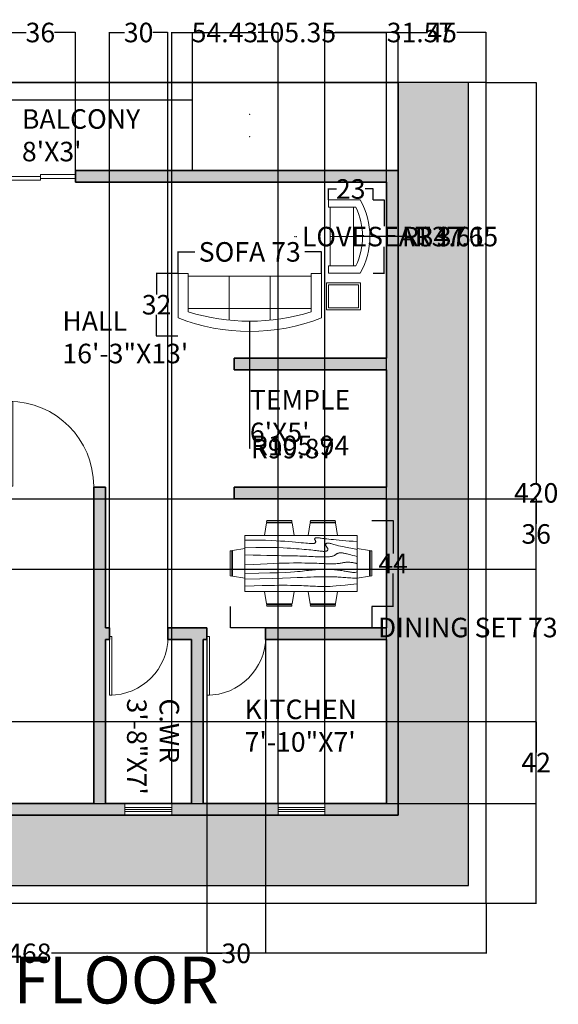
# Model space of a CAD drawing. Units: inches. Extents: x 377 to 1481, y 110 to 618.
# Tile 3 of 3: x 1205 to 1481, y 114 to 618. Entities that reach past the tile are written whole.
import ezdxf

# ---------------------------------------------------------------- set-up
doc = ezdxf.new("R2010")
doc.units = ezdxf.units.IN
doc.header["$MEASUREMENT"] = 0
for name, color, linetype, lineweight in [('A-ANNO-DIMS', 2, 'Continuous', 18), ('A-ANNO-TITL', 7, 'Continuous', 35), ('A-AREA-IDEN', 7, 'Continuous', 18), ('A-DOOR', 4, 'Continuous', 18), ('A-FLOR-BALC', 7, 'Continuous', 25), ('A-FURN', 8, 'Continuous', 18), ('A-GLAZ', 4, 'Continuous', 18), ('A-WALL', 7, 'Continuous', 35), ('C-PROP', 7, 'Continuous', 25)]:
    doc.layers.add(name, color=color, linetype=linetype, lineweight=lineweight)
doc.layers.add('A-WALL-PATT', color=251, linetype='Continuous', lineweight=13, true_color=0x636466)
doc.layers.add('L-PLNT-PATT', color=85, linetype='Continuous', lineweight=13, true_color=0x58ba48)
doc.styles.get("Standard").update_dxf_attribs({"font": 'arial.ttf'})
doc.dimstyles.get("Standard").update_dxf_attribs({"dimtxt": 10, "dimasz": 0.18, "dimexe": 0.18, "dimexo": 0.0625, "dimgap": 0.09, "dimtad": 0, "dimtih": 1, "dimtoh": 1, "dimdec": 0, "dimzin": 0, "dimdsep": 46, "dimlunit": 3, "dimtxsty": 'Standard', "dimcen": 0.09, "dimadec": 0, "dimazin": 0, "dimtfac": 1, "dimtdec": 0, "dimtofl": 0, "dimtmove": 0, "dimatfit": 3, "dimfxl": 1, "dimtolj": 1, "dimtzin": 0, "dimarcsym": 0})

# ---------------------------------------------------------------- blocks, each defined once
blk = doc.blocks.new('*U3')
for p, q in [((0, 0), (0, -6)), ((-40, 0), (-40, -6))]:
    blk.add_line(p, q)
blk.add_lwpolyline([(0, 0), (0, 40), (-1.75, 40), (-1.75, 0)], close=True)
blk.add_arc((0, 0), 40, 90, 180)
blk = doc.blocks.new('*U2')
for p, q in [((-40, 0), (-40, 6)), ((0, 0), (0, 6))]:
    blk.add_line(p, q)
blk.add_lwpolyline([(0, 0), (0, -40), (-1.75, -40), (-1.75, 0)], close=True)
blk.add_arc((0, 0), 40, 180, 270)
blk = doc.blocks.new('Sofa - Roundback 7 ft.')
for p, q in [((-36.000027, -34), (-36.000027, -11.4696)), ((-12.00002, -32.4421), (-12.00003, -6.5971)), ((11.99997, -32.4421), (11.99998, -6.5971)), ((35.99998, -34), (35.99998, -11.4696)), ((-35.999844, -13.3819), (35.9998, -13.3819)), ((-36.000027, -32.4421), (35.99998, -32.4421))]:
    blk.add_line(p, q)
for points in [[(-36.000027, -34), (-42.000027, -34), (-42.000027, -8)], [(41.99998, -8), (41.99998, -34), (35.99998, -34)]]:
    blk.add_lwpolyline(points)
for centre, radius, start, end in [((0, -114.25), 114.25, 68.43141, 111.5686), ((-0.00001, -127.1968), 121.1968, 72.72033, 107.2797)]:
    blk.add_arc(centre, radius, start, end)
blk = doc.blocks.new('Sofa - Roundback Loveseat 5 ft.')
for p, q in [((0, -32.44198), (0, -5.99998)), ((-24, -33.99998), (-24, -11.46958)), ((-23.9998, -13.38178), (23.99986, -13.38178)), ((24.00004, -33.99998), (24.00004, -11.46958)), ((-24, -32.44198), (24.00004, -32.44198))]:
    blk.add_line(p, q)
for points in [[(-24, -33.99998), (-30, -33.99998), (-30, -7.99998)], [(30.00004, -7.99998), (30.00004, -33.99998), (24.00004, -33.99998)]]:
    blk.add_lwpolyline(points)
for centre, radius, start, end in [((0, -60.24998), 60.24998, 60.13715, 119.8628), ((0, -61.38438), 55.38444, 64.32083, 115.6792)]:
    blk.add_arc(centre, radius, start, end)
blk = doc.blocks.new('Dining Set - 36 x 72 in.')
for p, q in [((-22.2343, 26.00059), (-23.4847, 17.99762)), ((-22.2304, 26), (-5.7608, 26)), ((-22, 27.5), (-22.1562, 26.50042)), ((-5.8416, 26.5), (-22.1534, 26.5)), ((-22, 27.5), (-6, 27.5)), ((-5.8437, 26.49966), (-6, 27.5)), ((-4.5152, 17.99762), (-5.7655, 25.99926)), ((5.7657, 26.00059), (4.5153, 17.99762)), ((5.7696, 26), (22.2392, 26)), ((6, 27.5), (5.8438, 26.50042)), ((22.1584, 26.5), (5.8466, 26.5)), ((6, 27.5), (22, 27.5)), ((22.1563, 26.49966), (22, 27.5)), ((23.4848, 17.99762), (22.2345, 25.99926)), ((36, 18), (-36, 18)), ((-36, 18), (-36, -18)), ((36, -18), (36, 18)), ((-45.5, 8), (-44.5004, 8.15617)), ((-45.5, 8), (-45.5, -8)), ((-44.5, -8.15843), (-44.5, 8.15338)), ((-44.0006, 8.23428), (-35.9976, 9.48474)), ((-44, 8.23041), (-44, -8.23915)), ((44.0006, 8.23428), (35.9976, 9.48474)), ((44, 8.23041), (44, -8.23915)), ((44.5, -8.15843), (44.5, 8.15338)), ((45.5, 8), (44.5005, 8.15617)), ((45.5, 8), (45.5, -8)), ((-44.4997, -8.15631), (-45.5, -8)), ((-35.9976, -9.48476), (-43.9993, -8.2345)), ((35.9976, -9.48476), (43.9993, -8.2345)), ((44.4997, -8.15631), (45.5, -8)), ((-36, -18), (36, -18)), ((-22.2343, -26.0006), (-23.4847, -17.99762)), ((-4.5152, -17.99762), (-5.7655, -25.99928)), ((5.7657, -26.0006), (4.5153, -17.99762)), ((23.4848, -17.99762), (22.2345, -25.99928)), ((-22.2304, -26), (-5.7608, -26)), ((-22, -27.5), (-22.1562, -26.50044)), ((-5.8416, -26.5), (-22.1534, -26.5)), ((-22, -27.5), (-6, -27.5)), ((-5.8437, -26.49967), (-6, -27.5)), ((5.7696, -26), (22.2392, -26)), ((6, -27.5), (5.8438, -26.50044)), ((22.1584, -26.5), (5.8466, -26.5)), ((6, -27.5), (22, -27.5)), ((22.1563, -26.49967), (22, -27.5))]:
    blk.add_line(p, q)
for points in [[(-36, 15), (-31.1772, 14.97754), (-26.8079, 14.91406), (-22.8538, 14.81543), (-19.276, 14.6875), (-16.0362, 14.53613), (-13.0957, 14.36718), (-10.4159, 14.18652), (-7.9583, 14), (-5.6904, 13.81315), (-3.6035, 13.63021), (-1.6954, 13.45508), (0.0365, 13.29166), (1.5945, 13.14388), (2.9811, 13.01562), (4.1988, 12.9108), (5.25, 12.83333), (6.1393, 12.78613), (6.8802, 12.76823), (7.4883, 12.77767), (7.9792, 12.8125), (8.3685, 12.87077), (8.6719, 12.95052), (8.9049, 13.0498), (9.0833, 13.16666), (9.2205, 13.29899), (9.3216, 13.44401), (9.3895, 13.59879), (9.4271, 13.76041), (9.4373, 13.92594), (9.4232, 14.09245), (9.3875, 14.257), (9.3333, 14.41666), (9.2638, 14.56917), (9.1836, 14.71484), (9.0975, 14.85465), (9.0104, 14.98958), (8.9272, 15.1206), (8.8529, 15.2487), (8.7922, 15.37483), (8.75, 15.5), (8.7305, 15.62467), (8.7344, 15.74739), (8.7617, 15.86621), (8.8125, 15.97916), (8.8867, 16.08431), (8.9844, 16.17968), (9.1055, 16.26334), (9.25, 16.33333), (9.4189, 16.38802), (9.6172, 16.42708), (9.8506, 16.45052), (10.125, 16.45833), (10.4463, 16.45052), (10.8203, 16.42708), (11.2529, 16.38802), (11.75, 16.33333), (12.3184, 16.26318), (12.9694, 16.17838), (13.7151, 16.07991), (14.5677, 15.96875), (15.5395, 15.84586), (16.6426, 15.71224), (17.8893, 15.56884), (19.2917, 15.41666), (20.859, 15.25667), (22.5879, 15.08984), (24.4721, 14.91715), (26.5052, 14.73958), (28.6809, 14.5581), (30.9929, 14.3737), (33.4347, 14.18733), (36, 14)], [(-36, 10), (-28.9766, 10.14274), (-23.1725, 10.20442), (-18.4241, 10.19775), (-14.5677, 10.13541), (-11.4399, 10.03011), (-8.877, 9.89453), (-6.7154, 9.74137), (-4.7917, 9.58333), (-2.9698, 9.43082), (-1.2246, 9.28515), (0.4415, 9.14534), (2.026, 9.01041), (3.5266, 8.87939), (4.9408, 8.7513), (6.266, 8.62516), (7.5, 8.5), (8.6411, 8.37549), (9.6914, 8.2539), (10.6538, 8.13818), (11.5312, 8.03125), (12.3267, 7.93603), (13.043, 7.85547), (13.6831, 7.79248), (14.25, 7.75), (14.7471, 7.7303), (15.1797, 7.73307), (15.5537, 7.75732), (15.875, 7.80208), (16.1494, 7.86637), (16.3828, 7.94922), (16.5811, 8.04964), (16.75, 8.16666), (16.8944, 8.29915), (17.0143, 8.44531), (17.1089, 8.60319), (17.1771, 8.77083), (17.218, 8.94629), (17.2305, 9.1276), (17.2137, 9.31282), (17.1667, 9.5), (17.0895, 9.6875), (16.987, 9.875), (16.8649, 10.0625), (16.7292, 10.25), (16.5856, 10.4375), (16.4401, 10.625), (16.2985, 10.8125), (16.1667, 11), (16.05, 11.18733), (15.9518, 11.3737), (15.8752, 11.5581), (15.8229, 11.73958), (15.798, 11.91715), (15.8034, 12.08984), (15.842, 12.25667), (15.9167, 12.41666), (16.0295, 12.56836), (16.1784, 12.70833), (16.3605, 12.83268), (16.5729, 12.9375), (16.8127, 13.01888), (17.0768, 13.07291), (17.3625, 13.0957), (17.6667, 13.08333), (17.9894, 13.03312), (18.3418, 12.94726), (18.7382, 12.82918), (19.1927, 12.68229), (19.7195, 12.51001), (20.3327, 12.31575), (21.0465, 12.10294), (21.875, 11.875), (22.8357, 11.63354), (23.959, 11.37304), (25.2786, 11.08618), (26.8282, 10.76562), (28.6414, 10.40405), (30.752, 9.99414), (33.1936, 9.52856), (36, 9)], [(-36, 5.5), (-30.7157, 5.3348), (-26.069, 5.20963), (-21.9946, 5.11767), (-18.4271, 5.05208), (-15.3009, 5.00602), (-12.5508, 4.97265), (-10.1112, 4.94515), (-7.9167, 4.91666), (-5.909, 4.88167), (-4.0586, 4.83984), (-2.3429, 4.79215), (-0.7396, 4.73958), (0.7739, 4.6831), (2.22, 4.6237), (3.6213, 4.56233), (5, 4.5), (6.373, 4.43782), (7.7344, 4.3776), (9.0723, 4.32129), (10.375, 4.27083), (11.6309, 4.22819), (12.8281, 4.19531), (13.9551, 4.17415), (15, 4.16666), (15.954, 4.17448), (16.819, 4.19791), (17.6001, 4.23698), (18.3021, 4.29166), (18.9299, 4.36198), (19.4883, 4.44791), (19.9823, 4.54948), (20.4167, 4.66666), (20.7969, 4.79899), (21.1302, 4.94401), (21.4245, 5.09879), (21.6875, 5.26041), (21.9271, 5.42594), (22.1511, 5.59245), (22.3672, 5.757), (22.5834, 5.91666), (22.8065, 6.06868), (23.0404, 6.21093), (23.2879, 6.34147), (23.5521, 6.45833), (23.8358, 6.55957), (24.142, 6.64323), (24.4735, 6.70735), (24.8334, 6.75), (25.2235, 6.76969), (25.642, 6.76692), (26.0858, 6.74267), (26.5521, 6.69791), (27.0379, 6.63362), (27.5404, 6.55078), (28.0565, 6.45036), (28.5834, 6.33333), (29.1242, 6.19987), (29.7071, 6.04687), (30.3661, 5.87044), (31.1354, 5.66666), (32.0493, 5.43164), (33.142, 5.16146), (34.4475, 4.85221), (36, 4.5)], [(-36, -1), (-30.7915, -0.6591), (-26.0195, -0.38216), (-21.6519, -0.16284), (-17.6563, 0.00521), (-14.0005, 0.12833), (-10.6523, 0.21289), (-7.5796, 0.26522), (-4.75, 0.29166), (-2.134, 0.29793), (0.2878, 0.28711), (2.5317, 0.26163), (4.6146, 0.22396), (6.5529, 0.17651), (8.3633, 0.12174), (10.0623, 0.06209), (11.6667, 0), (13.1899, -0.06201), (14.6341, -0.1211), (15.9982, -0.17432), (17.2813, -0.21875), (18.4823, -0.25147), (19.6003, -0.26953), (20.6343, -0.27002), (21.5834, -0.25), (22.4481, -0.20768), (23.2357, -0.14584), (23.9549, -0.06836), (24.6146, 0.02083), (25.2235, 0.11784), (25.7904, 0.21875), (26.3241, 0.31966), (26.8334, 0.41666), (27.3265, 0.50618), (27.8099, 0.58593), (28.2894, 0.65397), (28.7709, 0.70833), (29.2601, 0.74707), (29.763, 0.76823), (30.2855, 0.76985), (30.8334, 0.75), (31.4088, 0.70784), (31.9994, 0.64713), (32.589, 0.57275), (33.1615, 0.48958), (33.7008, 0.4025), (34.1908, 0.3164), (34.6153, 0.23616), (34.9584, 0.16666), (35.2099, 0.11165), (35.3848, 0.07031), (35.504, 0.04069), (35.5886, 0.02083), (35.6594, 0.00879), (35.7377, 0.0026), (35.8442, 0.00032), (36, 0)], [(-36, -6.5), (-27.1843, -6.31267), (-20.084, -6.1263), (-14.469, -5.9419), (-10.1094, -5.76042), (-6.7752, -5.58285), (-4.2363, -5.41016), (-2.2629, -5.24333), (-0.625, -5.08334), (0.8708, -4.93099), (2.2715, -4.78646), (3.5872, -4.64974), (4.8281, -4.52084), (6.0046, -4.39974), (7.127, -4.28646), (8.2053, -4.18099), (9.25, -4.08334), (10.2705, -3.99382), (11.2734, -3.91407), (12.2647, -3.84603), (13.25, -3.79167), (14.2354, -3.75293), (15.2266, -3.73177), (16.2295, -3.73015), (17.25, -3.75), (18.2912, -3.79248), (19.3451, -3.85547), (20.4009, -3.93604), (21.4479, -4.03125), (22.4754, -4.13819), (23.4727, -4.25391), (24.4289, -4.37549), (25.3334, -4.5), (26.1785, -4.62492), (26.9694, -4.74935), (27.7145, -4.87281), (28.4219, -4.99479), (29.1, -5.11483), (29.7572, -5.23242), (30.4016, -5.34709), (31.0417, -5.45834), (31.6837, -5.56437), (32.3262, -5.65821), (32.9658, -5.73153), (33.599, -5.77604), (34.2224, -5.78345), (34.8327, -5.74545), (35.4264, -5.65373), (36, -5.5)], [(-36, -10), (-26.4022, -9.81299), (-18.4675, -9.62891), (-11.9839, -9.45069), (-6.7396, -9.28125), (-2.5226, -9.12354), (0.8789, -8.98047), (3.6769, -8.85498), (6.0833, -8.75), (8.2767, -8.66765), (10.3021, -8.60677), (12.1712, -8.56543), (13.8958, -8.54167), (15.4876, -8.53353), (16.9583, -8.53907), (18.3197, -8.55632), (19.5834, -8.58334), (20.7616, -8.61841), (21.8685, -8.66081), (22.9188, -8.71004), (23.9271, -8.76563), (24.9081, -8.82707), (25.8763, -8.89388), (26.8465, -8.96558), (27.8334, -9.04167), (28.8474, -9.12118), (29.8828, -9.20117), (30.93, -9.27824), (31.9792, -9.34896), (33.0205, -9.40991), (34.0443, -9.45768), (35.0407, -9.48885), (36, -9.5)], [(-36, -14.5), (-30.0881, -14.33513), (-25.0332, -14.21224), (-20.7312, -14.12647), (-17.0781, -14.07292), (-13.97, -14.04671), (-11.3027, -14.04297), (-8.9724, -14.05681), (-6.875, -14.08334), (-4.9224, -14.11833), (-3.0905, -14.16016), (-1.3709, -14.20785), (0.2448, -14.26042), (1.7647, -14.3169), (3.1973, -14.3763), (4.5507, -14.43767), (5.8333, -14.5), (7.0554, -14.5621), (8.235, -14.62175), (9.3922, -14.67652), (10.5469, -14.72396), (11.7192, -14.76164), (12.929, -14.78711), (14.1965, -14.79794), (15.5417, -14.79167), (16.9933, -14.76424), (18.6152, -14.70508), (20.4804, -14.60197), (22.6615, -14.44271), (25.2312, -14.21509), (28.2624, -13.9069), (31.8277, -13.50594), (36, -13)]]:
    blk.add_lwpolyline(points)
blk = doc.blocks.new('WIN-24IN')
for p, q in [((0, 6), (0, 0)), ((24, 6), (24, 0)), ((24, 4), (0, 4)), ((24, 3), (0, 3)), ((24, 2), (0, 2))]:
    blk.add_line(p, q)
blk = doc.blocks.new('*D21')
at = {"layer": 'A-ANNO-DIMS', "color": 0, "lineweight": -2, "transparency": 16777216}
for p, q in [((1285.78, 488.24), (1285.78, 499.38)), ((1285.96, 499.2), (1294.31, 499.2)), ((1359.03, 499.2), (1350.68, 499.2)), ((1359.21, 488.24), (1359.21, 499.38))]:
    blk.add_line(p, q, dxfattribs=at)
at = {"layer": 'A-ANNO-DIMS', "color": 0, "lineweight": 100, "transparency": 16777216}
for points in [[(1285.96, 499.23), (1285.96, 499.17), (1285.78, 499.2)], [(1359.03, 499.23), (1359.03, 499.17), (1359.21, 499.2)]]:
    blk.add_solid(points, dxfattribs=at)
at = {"layer": 'Defpoints', "color": 0, "lineweight": 100, "transparency": 16777216}
for p in [(1285.78, 499.2), (1285.78, 488.18), (1359.21, 488.18)]:
    blk.add_point(p, dxfattribs=at)
at = {"layer": 'A-ANNO-DIMS', "color": 0, "transparency": 16777216, "insert": (1322.49, 499.2), "char_height": 10, "attachment_point": 5}
blk.add_mtext('\\A1;SOFA 73', dxfattribs=at)
blk = doc.blocks.new('*D22')
at = {"layer": 'A-ANNO-DIMS', "color": 0, "lineweight": -2, "transparency": 16777216}
for p, q in [((1285.72, 488.18), (1274.59, 488.18)), ((1274.77, 488), (1274.77, 477.35)), ((1274.77, 456.31), (1274.77, 466.96)), ((1285.72, 456.13), (1274.59, 456.13))]:
    blk.add_line(p, q, dxfattribs=at)
at = {"layer": 'A-ANNO-DIMS', "color": 0, "lineweight": 100, "transparency": 16777216}
for points in [[(1274.74, 488), (1274.8, 488), (1274.77, 488.18)], [(1274.74, 456.31), (1274.8, 456.31), (1274.77, 456.13)]]:
    blk.add_solid(points, dxfattribs=at)
at = {"layer": 'Defpoints', "color": 0, "lineweight": 100, "transparency": 16777216}
for p in [(1285.78, 488.18), (1274.77, 456.13), (1285.78, 456.13)]:
    blk.add_point(p, dxfattribs=at)
at = {"layer": 'A-ANNO-DIMS', "color": 0, "transparency": 16777216, "insert": (1274.77, 472.16), "char_height": 10, "attachment_point": 5}
blk.add_mtext('\\A1;32', dxfattribs=at)
blk = doc.blocks.new('*D23')
at = {"layer": 'A-ANNO-DIMS', "color": 0, "lineweight": -2, "transparency": 16777216}
for p, q in [((1385.75, 525.79), (1391.49, 525.79)), ((1391.31, 525.61), (1391.31, 512.31)), ((1391.31, 488.47), (1391.31, 501.77)), ((1385.75, 488.29), (1391.49, 488.29))]:
    blk.add_line(p, q, dxfattribs=at)
at = {"layer": 'A-ANNO-DIMS', "color": 0, "lineweight": 100, "transparency": 16777216}
for points in [[(1391.28, 525.61), (1391.34, 525.61), (1391.31, 525.79)], [(1391.28, 488.47), (1391.34, 488.47), (1391.31, 488.29)]]:
    blk.add_solid(points, dxfattribs=at)
at = {"layer": 'Defpoints', "color": 0, "lineweight": 100, "transparency": 16777216}
for p in [(1385.68, 525.79), (1385.68, 488.29), (1391.31, 488.29)]:
    blk.add_point(p, dxfattribs=at)
at = {"layer": 'A-ANNO-DIMS', "color": 0, "transparency": 16777216, "insert": (1391.31, 507.04), "char_height": 10, "attachment_point": 5}
blk.add_mtext('\\A1;LOVESEAT 37', dxfattribs=at)
blk = doc.blocks.new('*D24')
at = {"layer": 'A-ANNO-DIMS', "color": 0, "lineweight": -2, "transparency": 16777216}
for p, q in [((1362.77, 525.85), (1362.77, 531.59)), ((1362.95, 531.41), (1366.89, 531.41)), ((1385.5, 531.41), (1381.56, 531.41)), ((1385.68, 525.85), (1385.68, 531.59))]:
    blk.add_line(p, q, dxfattribs=at)
at = {"layer": 'A-ANNO-DIMS', "color": 0, "lineweight": 100, "transparency": 16777216}
for points in [[(1362.95, 531.44), (1362.95, 531.38), (1362.77, 531.41)], [(1385.5, 531.44), (1385.5, 531.38), (1385.68, 531.41)]]:
    blk.add_solid(points, dxfattribs=at)
at = {"layer": 'Defpoints', "color": 0, "lineweight": 100, "transparency": 16777216}
for p in [(1385.68, 531.41), (1362.77, 525.79), (1385.68, 525.79)]:
    blk.add_point(p, dxfattribs=at)
at = {"layer": 'A-ANNO-DIMS', "color": 0, "transparency": 16777216, "insert": (1374.23, 531.41), "char_height": 10, "attachment_point": 5}
blk.add_mtext('\\A1;23', dxfattribs=at)
blk = doc.blocks.new('*D25')
at = {"layer": 'A-ANNO-DIMS', "color": 0, "lineweight": -2, "transparency": 16777216}
for p, q in [((1312.48, 317.75), (1312.48, 306.75)), ((1385.06, 317.75), (1385.06, 306.75)), ((1312.66, 306.93), (1384.88, 306.93)), ((1385.06, 306.93), (1385.24, 306.93))]:
    blk.add_line(p, q, dxfattribs=at)
at = {"layer": 'A-ANNO-DIMS', "color": 0, "lineweight": 100, "transparency": 16777216}
for points in [[(1312.66, 306.96), (1312.66, 306.9), (1312.48, 306.93)], [(1384.88, 306.96), (1384.88, 306.9), (1385.06, 306.93)]]:
    blk.add_solid(points, dxfattribs=at)
at = {"layer": 'Defpoints', "color": 0, "lineweight": 100, "transparency": 16777216}
for p in [(1312.48, 317.81), (1385.06, 317.81), (1385.06, 306.93)]:
    blk.add_point(p, dxfattribs=at)
at = {"layer": 'A-ANNO-DIMS', "color": 0, "transparency": 16777216, "insert": (1434.16, 306.93), "char_height": 10, "attachment_point": 5}
blk.add_mtext('\\A1;DINING SET 73', dxfattribs=at)
blk = doc.blocks.new('*D26')
at = {"layer": 'A-ANNO-DIMS', "color": 0, "lineweight": -2, "transparency": 16777216}
for p, q in [((1385.12, 361.68), (1396.13, 361.68)), ((1395.95, 361.5), (1395.95, 344.84)), ((1395.95, 317.99), (1395.95, 334.66)), ((1385.12, 317.81), (1396.13, 317.81))]:
    blk.add_line(p, q, dxfattribs=at)
at = {"layer": 'A-ANNO-DIMS', "color": 0, "lineweight": 100, "transparency": 16777216}
for points in [[(1395.92, 361.5), (1395.98, 361.5), (1395.95, 361.68)], [(1395.92, 317.99), (1395.98, 317.99), (1395.95, 317.81)]]:
    blk.add_solid(points, dxfattribs=at)
at = {"layer": 'Defpoints', "color": 0, "lineweight": 100, "transparency": 16777216}
for p in [(1385.06, 361.68), (1395.95, 361.68), (1385.06, 317.81)]:
    blk.add_point(p, dxfattribs=at)
at = {"layer": 'A-ANNO-DIMS', "color": 0, "transparency": 16777216, "insert": (1395.95, 339.75), "char_height": 10, "attachment_point": 5}
blk.add_mtext('\\A1;44', dxfattribs=at)
blk = doc.blocks.new('*D40')
at = {"layer": 'A-ANNO-DIMS', "color": 0, "lineweight": -2, "transparency": 16777216}
for p, q in [((975.57, 165.78), (975.57, 140.01)), ((1443.57, 165.78), (1443.57, 140.01)), ((975.75, 140.19), (1198.22, 140.19)), ((1443.39, 140.19), (1220.92, 140.19))]:
    blk.add_line(p, q, dxfattribs=at)
at = {"layer": 'A-ANNO-DIMS', "color": 0, "lineweight": 100, "transparency": 16777216}
for points in [[(975.75, 140.22), (975.75, 140.16), (975.57, 140.19)], [(1443.39, 140.22), (1443.39, 140.16), (1443.57, 140.19)]]:
    blk.add_solid(points, dxfattribs=at)
at = {"layer": 'Defpoints', "color": 0, "lineweight": 100, "transparency": 16777216}
for p in [(975.57, 165.84), (1443.57, 165.84), (1443.57, 140.19)]:
    blk.add_point(p, dxfattribs=at)
at = {"layer": 'A-ANNO-DIMS', "color": 0, "transparency": 16777216, "insert": (1209.57, 140.19), "char_height": 10, "attachment_point": 5}
blk.add_mtext('\\A1;468', dxfattribs=at)
blk = doc.blocks.new('*D41')
at = {"layer": 'A-ANNO-DIMS', "color": 0, "lineweight": -2, "transparency": 16777216}
for p, q in [((1443.63, 585.84), (1469.4, 585.84)), ((1469.22, 585.66), (1469.22, 381.04)), ((1469.22, 166.02), (1469.22, 370.64)), ((1443.63, 165.84), (1469.4, 165.84))]:
    blk.add_line(p, q, dxfattribs=at)
at = {"layer": 'A-ANNO-DIMS', "color": 0, "lineweight": 100, "transparency": 16777216}
for points in [[(1469.19, 585.66), (1469.25, 585.66), (1469.22, 585.84)], [(1469.19, 166.02), (1469.25, 166.02), (1469.22, 165.84)]]:
    blk.add_solid(points, dxfattribs=at)
at = {"layer": 'Defpoints', "color": 0, "lineweight": 100, "transparency": 16777216}
for p in [(1443.57, 585.84), (1469.22, 585.84), (1443.57, 165.84)]:
    blk.add_point(p, dxfattribs=at)
at = {"layer": 'A-ANNO-DIMS', "color": 0, "transparency": 16777216, "insert": (1469.22, 375.84), "char_height": 10, "attachment_point": 5}
blk.add_mtext('\\A1;420', dxfattribs=at)
blk = doc.blocks.new('*D44')
at = {"layer": 'A-ANNO-DIMS', "color": 0, "lineweight": -2, "transparency": 16777216}
for p, q in [((1293.22, 540.9), (1293.22, 611.67)), ((1293.4, 611.49), (1325.48, 611.49)), ((1398.39, 611.49), (1366.31, 611.49)), ((1398.57, 540.9), (1398.57, 611.67))]:
    blk.add_line(p, q, dxfattribs=at)
at = {"layer": 'A-ANNO-DIMS', "color": 0, "lineweight": 100, "transparency": 16777216}
for points in [[(1293.4, 611.52), (1293.4, 611.46), (1293.22, 611.49)], [(1398.39, 611.52), (1398.39, 611.46), (1398.57, 611.49)]]:
    blk.add_solid(points, dxfattribs=at)
at = {"layer": 'Defpoints', "color": 0, "lineweight": 100, "transparency": 16777216}
for p in [(1398.57, 611.49), (1293.22, 540.84), (1398.57, 540.84)]:
    blk.add_point(p, dxfattribs=at)
at = {"layer": 'A-ANNO-DIMS', "color": 0, "transparency": 16777216, "insert": (1345.9, 611.49), "char_height": 10, "attachment_point": 5}
blk.add_mtext('\\A1;105.35', dxfattribs=at)
blk = doc.blocks.new('*D45')
at = {"layer": 'A-ANNO-DIMS', "color": 0, "lineweight": -2, "transparency": 16777216}
for p, q in [((1398.57, 585.9), (1398.57, 611.67)), ((1398.75, 611.49), (1413.58, 611.49)), ((1443.39, 611.49), (1428.56, 611.49)), ((1443.57, 585.9), (1443.57, 611.67))]:
    blk.add_line(p, q, dxfattribs=at)
at = {"layer": 'A-ANNO-DIMS', "color": 0, "lineweight": 100, "transparency": 16777216}
for points in [[(1398.75, 611.52), (1398.75, 611.46), (1398.57, 611.49)], [(1443.39, 611.52), (1443.39, 611.46), (1443.57, 611.49)]]:
    blk.add_solid(points, dxfattribs=at)
at = {"layer": 'Defpoints', "color": 0, "lineweight": 100, "transparency": 16777216}
for p in [(1443.57, 611.49), (1398.57, 585.84), (1443.57, 585.84)]:
    blk.add_point(p, dxfattribs=at)
at = {"layer": 'A-ANNO-DIMS', "color": 0, "transparency": 16777216, "insert": (1421.07, 611.49), "char_height": 10, "attachment_point": 5}
blk.add_mtext('\\A1;45', dxfattribs=at)
blk = doc.blocks.new('*D48')
at = {"layer": 'A-ANNO-DIMS', "color": 0, "lineweight": -2, "transparency": 16777216}
for p, q in [((1361, 216.9), (1361, 611.67)), ((1361.18, 611.49), (1392.39, 611.49)), ((1392.57, 216.9), (1392.57, 611.67)), ((1392.57, 611.49), (1392.75, 611.49))]:
    blk.add_line(p, q, dxfattribs=at)
at = {"layer": 'A-ANNO-DIMS', "color": 0, "lineweight": 100, "transparency": 16777216}
for points in [[(1361.18, 611.52), (1361.18, 611.46), (1361, 611.49)], [(1392.39, 611.52), (1392.39, 611.46), (1392.57, 611.49)]]:
    blk.add_solid(points, dxfattribs=at)
at = {"layer": 'Defpoints', "color": 0, "lineweight": 100, "transparency": 16777216}
for p in [(1392.57, 611.49), (1361, 216.84), (1392.57, 216.84)]:
    blk.add_point(p, dxfattribs=at)
at = {"layer": 'A-ANNO-DIMS', "color": 0, "transparency": 16777216, "insert": (1409.71, 611.49), "char_height": 10, "attachment_point": 5}
blk.add_mtext('\\A1;31.57', dxfattribs=at)
blk = doc.blocks.new('*D49')
at = {"layer": 'A-ANNO-DIMS', "color": 0, "lineweight": -2, "transparency": 16777216}
for p, q in [((1282.57, 216.9), (1282.57, 611.67)), ((1282.75, 611.49), (1292.82, 611.49)), ((1336.82, 611.49), (1326.75, 611.49)), ((1337, 216.9), (1337, 611.67))]:
    blk.add_line(p, q, dxfattribs=at)
at = {"layer": 'A-ANNO-DIMS', "color": 0, "lineweight": 100, "transparency": 16777216}
for points in [[(1282.75, 611.52), (1282.75, 611.46), (1282.57, 611.49)], [(1336.82, 611.52), (1336.82, 611.46), (1337, 611.49)]]:
    blk.add_solid(points, dxfattribs=at)
at = {"layer": 'Defpoints', "color": 0, "lineweight": 100, "transparency": 16777216}
for p in [(1337, 611.49), (1282.57, 216.84), (1337, 216.84)]:
    blk.add_point(p, dxfattribs=at)
at = {"layer": 'A-ANNO-DIMS', "color": 0, "transparency": 16777216, "insert": (1309.78, 611.49), "char_height": 10, "attachment_point": 5}
blk.add_mtext('\\A1;54.43', dxfattribs=at)
blk = doc.blocks.new('*D50')
at = {"layer": 'A-ANNO-DIMS', "color": 0, "lineweight": -2, "transparency": 16777216}
for p, q in [((1250.57, 306.9), (1250.57, 611.67)), ((1250.75, 611.49), (1258.34, 611.49)), ((1280.39, 611.49), (1272.8, 611.49)), ((1280.57, 306.9), (1280.57, 611.67))]:
    blk.add_line(p, q, dxfattribs=at)
at = {"layer": 'A-ANNO-DIMS', "color": 0, "lineweight": 100, "transparency": 16777216}
for points in [[(1250.75, 611.52), (1250.75, 611.46), (1250.57, 611.49)], [(1280.39, 611.52), (1280.39, 611.46), (1280.57, 611.49)]]:
    blk.add_solid(points, dxfattribs=at)
at = {"layer": 'Defpoints', "color": 0, "lineweight": 100, "transparency": 16777216}
for p in [(1280.57, 611.49), (1250.57, 306.84), (1280.57, 306.84)]:
    blk.add_point(p, dxfattribs=at)
at = {"layer": 'A-ANNO-DIMS', "color": 0, "transparency": 16777216, "insert": (1265.57, 611.49), "char_height": 10, "attachment_point": 5}
blk.add_mtext('\\A1;30', dxfattribs=at)
blk = doc.blocks.new('*D51')
at = {"layer": 'A-ANNO-DIMS', "color": 0, "lineweight": -2, "transparency": 16777216}
for p, q in [((1300.57, 300.71), (1300.57, 140.01)), ((1330.57, 300.78), (1330.57, 140.01)), ((1300.75, 140.19), (1308.34, 140.19)), ((1330.39, 140.19), (1322.8, 140.19))]:
    blk.add_line(p, q, dxfattribs=at)
at = {"layer": 'A-ANNO-DIMS', "color": 0, "lineweight": 100, "transparency": 16777216}
for points in [[(1300.75, 140.22), (1300.75, 140.16), (1300.57, 140.19)], [(1330.39, 140.22), (1330.39, 140.16), (1330.57, 140.19)]]:
    blk.add_solid(points, dxfattribs=at)
at = {"layer": 'Defpoints', "color": 0, "lineweight": 100, "transparency": 16777216}
for p in [(1300.57, 300.77), (1330.57, 300.84), (1330.57, 140.19)]:
    blk.add_point(p, dxfattribs=at)
at = {"layer": 'A-ANNO-DIMS', "color": 0, "transparency": 16777216, "insert": (1315.57, 140.19), "char_height": 10, "attachment_point": 5}
blk.add_mtext('\\A1;30', dxfattribs=at)
blk = doc.blocks.new('*D53')
at = {"layer": 'A-ANNO-DIMS', "color": 0, "lineweight": -2, "transparency": 16777216}
for p, q in [((1197.22, 540.9), (1197.22, 611.67)), ((1197.4, 611.49), (1207.98, 611.49)), ((1233.04, 611.49), (1222.47, 611.49)), ((1233.22, 540.9), (1233.22, 611.67))]:
    blk.add_line(p, q, dxfattribs=at)
at = {"layer": 'A-ANNO-DIMS', "color": 0, "lineweight": 100, "transparency": 16777216}
for points in [[(1197.4, 611.52), (1197.4, 611.46), (1197.22, 611.49)], [(1233.04, 611.52), (1233.04, 611.46), (1233.22, 611.49)]]:
    blk.add_solid(points, dxfattribs=at)
at = {"layer": 'Defpoints', "color": 0, "lineweight": 100, "transparency": 16777216}
for p in [(1233.22, 611.49), (1197.22, 540.84), (1233.22, 540.84)]:
    blk.add_point(p, dxfattribs=at)
at = {"layer": 'A-ANNO-DIMS', "color": 0, "transparency": 16777216, "insert": (1215.22, 611.49), "char_height": 10, "attachment_point": 5}
blk.add_mtext('\\A1;36', dxfattribs=at)
blk = doc.blocks.new('*D56')
at = {"layer": 'A-ANNO-DIMS', "color": 0, "lineweight": -2, "transparency": 16777216}
for p, q in [((1137.29, 258.84), (1469.4, 258.84)), ((1469.22, 258.66), (1469.22, 242.95)), ((1469.22, 217.02), (1469.22, 232.73)), ((1137.29, 216.84), (1469.4, 216.84))]:
    blk.add_line(p, q, dxfattribs=at)
at = {"layer": 'A-ANNO-DIMS', "color": 0, "lineweight": 100, "transparency": 16777216}
for points in [[(1469.19, 258.66), (1469.25, 258.66), (1469.22, 258.84)], [(1469.19, 217.02), (1469.25, 217.02), (1469.22, 216.84)]]:
    blk.add_solid(points, dxfattribs=at)
at = {"layer": 'Defpoints', "color": 0, "lineweight": 100, "transparency": 16777216}
for p in [(1137.22, 258.84), (1469.22, 258.84), (1137.22, 216.84)]:
    blk.add_point(p, dxfattribs=at)
at = {"layer": 'A-ANNO-DIMS', "color": 0, "transparency": 16777216, "insert": (1469.22, 237.84), "char_height": 10, "attachment_point": 5}
blk.add_mtext('\\A1;42', dxfattribs=at)
blk = doc.blocks.new('*D57')
at = {"layer": 'A-ANNO-DIMS', "color": 0, "lineweight": -2, "transparency": 16777216}
for p, q in [((1137.29, 372.84), (1469.4, 372.84)), ((1469.22, 372.66), (1469.22, 360.04)), ((1469.22, 337.02), (1469.22, 349.64)), ((1137.29, 336.84), (1469.4, 336.84))]:
    blk.add_line(p, q, dxfattribs=at)
at = {"layer": 'A-ANNO-DIMS', "color": 0, "lineweight": 100, "transparency": 16777216}
for points in [[(1469.19, 372.66), (1469.25, 372.66), (1469.22, 372.84)], [(1469.19, 337.02), (1469.25, 337.02), (1469.22, 336.84)]]:
    blk.add_solid(points, dxfattribs=at)
at = {"layer": 'Defpoints', "color": 0, "lineweight": 100, "transparency": 16777216}
for p in [(1137.22, 372.84), (1469.22, 372.84), (1137.22, 336.84)]:
    blk.add_point(p, dxfattribs=at)
at = {"layer": 'A-ANNO-DIMS', "color": 0, "transparency": 16777216, "insert": (1469.22, 354.84), "char_height": 10, "attachment_point": 5}
blk.add_mtext('\\A1;36', dxfattribs=at)
blk = doc.blocks.new('*D59')
at = {"layer": 'A-ANNO-DIMS', "color": 0, "lineweight": -2, "transparency": 16777216}
for p, q in [((1322.4, 569.65), (1322.58, 569.65)), ((1322.49, 569.56), (1322.49, 569.74)), ((1322.49, 400.14), (1322.49, 463.53)), ((1322.68, 400.14), (1322.49, 400.14))]:
    blk.add_line(p, q, dxfattribs=at)
at = {"layer": 'A-ANNO-DIMS', "color": 0, "lineweight": 100, "transparency": 16777216}
blk.add_solid([(1322.53, 463.53), (1322.47, 463.53), (1322.49, 463.71)], dxfattribs=at)
at = {"layer": 'Defpoints', "color": 0, "lineweight": 100, "transparency": 16777216}
for p in [(1322.49, 569.65), (1322.49, 463.71)]:
    blk.add_point(p, dxfattribs=at)
at = {"layer": 'A-ANNO-DIMS', "color": 0, "transparency": 16777216, "insert": (1348.29, 400.14), "char_height": 10, "attachment_point": 5}
blk.add_mtext('\\A1;R105.94', dxfattribs=at)
blk = doc.blocks.new('*D60')
at = {"layer": 'A-ANNO-DIMS', "color": 0, "lineweight": -2, "transparency": 16777216}
for p, q in [((1322.4, 558.33), (1322.58, 558.33)), ((1322.49, 558.24), (1322.49, 558.42)), ((1322.49, 398.54), (1322.49, 458.28)), ((1322.68, 398.54), (1322.49, 398.54))]:
    blk.add_line(p, q, dxfattribs=at)
at = {"layer": 'A-ANNO-DIMS', "color": 0, "lineweight": 100, "transparency": 16777216}
blk.add_solid([(1322.53, 458.28), (1322.47, 458.28), (1322.49, 458.46)], dxfattribs=at)
at = {"layer": 'Defpoints', "color": 0, "lineweight": 100, "transparency": 16777216}
for p in [(1322.49, 558.33), (1322.49, 458.46)]:
    blk.add_point(p, dxfattribs=at)
at = {"layer": 'A-ANNO-DIMS', "color": 0, "transparency": 16777216, "insert": (1344.42, 398.54), "char_height": 10, "attachment_point": 5}
blk.add_mtext('\\A1;R99.87', dxfattribs=at)
blk = doc.blocks.new('*D61')
at = {"layer": 'A-ANNO-DIMS', "color": 0, "lineweight": -2, "transparency": 16777216}
for p, q in [((1346.28, 507.04), (1346.46, 507.04)), ((1346.37, 506.95), (1346.37, 507.13)), ((1406.61, 507.04), (1384.2, 507.04))]:
    blk.add_line(p, q, dxfattribs=at)
at = {"layer": 'A-ANNO-DIMS', "color": 0, "lineweight": 100, "transparency": 16777216}
blk.add_solid([(1384.2, 507.07), (1384.2, 507.01), (1384.02, 507.04)], dxfattribs=at)
at = {"layer": 'Defpoints', "color": 0, "lineweight": 100, "transparency": 16777216}
for p in [(1346.37, 507.04), (1384.02, 507.04)]:
    blk.add_point(p, dxfattribs=at)
at = {"layer": 'A-ANNO-DIMS', "color": 0, "transparency": 16777216, "insert": (1428.39, 507.04), "char_height": 10, "attachment_point": 5}
blk.add_mtext('\\A1;R37.65', dxfattribs=at)
blk = doc.blocks.new('*D62')
at = {"layer": 'A-ANNO-DIMS', "color": 0, "lineweight": -2, "transparency": 16777216}
for p, q in [((1345.57, 507.04), (1345.75, 507.04)), ((1345.66, 506.95), (1345.66, 507.13)), ((1401.04, 507.04), (1380.45, 507.04))]:
    blk.add_line(p, q, dxfattribs=at)
at = {"layer": 'A-ANNO-DIMS', "color": 0, "lineweight": 100, "transparency": 16777216}
blk.add_solid([(1380.45, 507.07), (1380.45, 507.01), (1380.27, 507.04)], dxfattribs=at)
at = {"layer": 'Defpoints', "color": 0, "lineweight": 100, "transparency": 16777216}
for p in [(1345.66, 507.04), (1380.27, 507.04)]:
    blk.add_point(p, dxfattribs=at)
at = {"layer": 'A-ANNO-DIMS', "color": 0, "transparency": 16777216, "insert": (1421.82, 507.04), "char_height": 10, "attachment_point": 5}
blk.add_mtext('\\A1;R34.61', dxfattribs=at)

msp = doc.modelspace()

# ---------------------------------------------------------------- hatches: boundary and pattern name
at = {"layer": 'A-WALL-PATT'}
h = msp.add_hatch(color=256, dxfattribs=at)
h.dxf.hatch_style = 1
h.paths.add_polyline_path([(1035.2247, 216.8394), (1035.2247, 372.8394), (1137.2247, 372.8394), (1197.2247, 372.8394), (1199.2247, 372.8394), (1199.2247, 378.8394), (1197.2247, 378.8394), (1197.2247, 496.8394), (1191.2247, 496.8394), (1191.2247, 378.8394), (1137.2247, 378.8394), (1035.2247, 378.8394), (1035.2247, 482.8394), (1137.2247, 482.8394), (1143.2247, 482.8394), (1143.2247, 502.8394), (1139.2247, 502.8394), (1139.2247, 486.8394), (1137.2247, 486.8394), (1035.2247, 486.8394), (1035.2247, 497.8925), (1029.2247, 497.8925), (1029.2247, 210.8394), (1258.5701, 210.8394), (1258.5701, 216.8394), (1248.5701, 216.8394), (1248.5701, 300.8394), (1250.5701, 300.8394), (1250.5701, 306.8394), (1248.5701, 306.8394), (1248.5701, 378.8394), (1242.5701, 378.8394), (1242.5701, 216.8394)])
h.paths.add_polyline_path([(1298.5701, 216.8394), (1298.5701, 300.8394), (1300.5689, 300.769), (1300.5689, 306.8394), (1298.5701, 306.8394), (1280.5701, 306.8394), (1280.5701, 300.8394), (1292.5701, 300.8394), (1292.5701, 216.8394), (1282.5701, 216.8394), (1282.5701, 210.8394), (1336.9971, 210.8394), (1336.9971, 216.8394)], flags=17)
h.paths.add_polyline_path([(1360.9971, 216.8394), (1360.9971, 210.8394), (1398.5701, 210.8394), (1398.5701, 540.8394), (1233.2247, 540.8394), (1233.2247, 534.8394), (1392.5701, 534.8394), (1392.5701, 444.8394), (1314.5701, 444.8394), (1314.5701, 438.8394), (1392.5701, 438.8394), (1392.5701, 378.8394), (1314.5701, 378.8394), (1314.5701, 372.8394), (1392.5701, 372.8394), (1392.5701, 306.8394), (1330.6485, 306.8394), (1330.6485, 302.3275, -0.01237335), (1330.6116, 300.8394), (1392.5701, 300.8394), (1392.5701, 216.8394)])
h.paths.add_polyline_path([(1029.2247, 540.8394), (1029.2247, 521.8925), (1035.2247, 521.8925), (1035.2247, 534.8394), (1137.2247, 534.8394), (1139.2247, 534.8394), (1139.2247, 532.8394), (1143.2247, 532.8394), (1143.2247, 534.8394), (1191.2247, 534.8394), (1191.2247, 532.8394), (1197.2247, 532.8394), (1197.2247, 534.8394), (1197.2247, 540.8394), (1137.2247, 540.8394)])
at = {"layer": 'L-PLNT-PATT'}
h = msp.add_hatch(color=256, dxfattribs=at)
h.dxf.hatch_style = 1
h.paths.add_polyline_path([(985.0991, 174.8394), (1434.5701, 174.8394), (1434.5701, 585.8394), (1398.5701, 585.8394), (1398.5701, 540.8394), (1398.5701, 210.8394), (1029.2247, 210.8394), (1029.2247, 540.8394), (1029.2247, 585.8394), (1008.5848, 585.8394)])

# ---------------------------------------------------------------- linework, layer by layer
at = {"layer": 'A-DOOR'}
for points in [[(1197.2247, 537.8394), (1197.2247, 535.8394), (1215.2247, 535.8394), (1215.2247, 537.8394)], [(1215.2247, 538.8394), (1215.2247, 536.8394), (1233.2247, 536.8394), (1233.2247, 538.8394)]]:
    msp.add_lwpolyline(points, close=True, dxfattribs=at)
at = {"layer": 'A-FLOR-BALC'}
for p, q in [((1029.2247, 585.8394), (1398.5701, 585.8394)), ((1293.2247, 540.8394), (1293.2247, 585.8394)), ((1398.5701, 585.8394), (1398.5701, 540.8394)), ((1293.2247, 576.8394), (1197.2247, 576.8394))]:
    msp.add_line(p, q, dxfattribs=at)
at = {"layer": 'A-FURN'}
for points in [[(1379.181, 469.6104), (1361.8546, 469.6104), (1361.8546, 483.4236), (1379.181, 483.4236)], [(1378.181, 470.6104), (1362.8546, 470.6104), (1362.8546, 482.4236), (1378.181, 482.4236)]]:
    msp.add_lwpolyline(points, close=True, dxfattribs=at)
at = {"layer": 'A-WALL'}
for p, q in [((1398.5701, 540.8394), (1233.2247, 540.8394)), ((1233.2247, 534.8394), (1233.2247, 540.8394)), ((1398.5701, 210.8394), (1398.5701, 540.8394)), ((1392.5701, 534.8394), (1233.2247, 534.8394)), ((1392.5701, 444.8394), (1392.5701, 534.8394)), ((1314.5701, 444.8394), (1392.5701, 444.8394)), ((1314.5701, 438.8394), (1314.5701, 444.8394)), ((1314.5701, 438.8394), (1392.5701, 438.8394)), ((1392.5701, 378.8394), (1392.5701, 438.8394)), ((1242.5701, 216.8394), (1242.5701, 378.8394)), ((1242.5701, 378.8394), (1248.5701, 378.8394)), ((1248.5701, 306.8394), (1248.5701, 378.8394)), ((1314.5701, 372.8394), (1314.5701, 378.8394)), ((1314.5701, 378.8394), (1392.5701, 378.8394)), ((1314.5701, 372.8394), (1392.5701, 372.8394)), ((1392.5701, 306.8394), (1392.5701, 372.8394)), ((1250.5701, 306.8394), (1248.5701, 306.8394)), ((1250.5701, 300.8394), (1250.5701, 306.8394)), ((1280.5701, 306.8394), (1298.5701, 306.8394)), ((1280.5701, 300.8394), (1280.5701, 306.8394)), ((1300.5689, 306.8394), (1298.5701, 306.8394)), ((1300.5689, 300.769), (1300.5689, 306.8394)), ((1330.5701, 300.8394), (1330.5701, 306.8394)), ((1330.5701, 306.8394), (1392.5701, 306.8394)), ((1248.5701, 216.8394), (1248.5701, 300.8394)), ((1248.5701, 300.8394), (1250.5701, 300.8394)), ((1280.5701, 300.8394), (1292.5701, 300.8394)), ((1292.5701, 216.8394), (1292.5701, 300.8394)), ((1298.5701, 216.8394), (1298.5701, 300.8394)), ((1298.5701, 300.8394), (1300.5689, 300.769)), ((1330.5701, 300.8394), (1392.5701, 300.8394)), ((1392.5701, 216.8394), (1392.5701, 300.8394)), ((1035.2247, 216.8394), (1242.5701, 216.8394)), ((1248.5701, 216.8394), (1292.5701, 216.8394)), ((1292.5701, 216.8394), (1248.5701, 216.8394)), ((1298.5701, 216.8394), (1392.5701, 216.8394)), ((1029.2247, 210.8394), (1398.5701, 210.8394))]:
    msp.add_line(p, q, dxfattribs=at)
at = {"layer": 'C-PROP'}
for p, q in [((1443.5701, 585.8394), (999.5701, 585.8394)), ((1434.5701, 174.8394), (1434.5701, 585.8394)), ((1443.5701, 165.8394), (1443.5701, 585.8394)), ((976.0844, 174.8394), (1434.5701, 174.8394)), ((975.5701, 165.8394), (1443.5701, 165.8394))]:
    msp.add_line(p, q, dxfattribs=at)

# ---------------------------------------------------------------- block references
at = {"layer": 'A-DOOR', "rotation": 180}
for name, p, xscale, yscale, zscale in [('*U2', (1199.2247, 379.3372), 1.082974319922984, 1.082974319922984, 1.082974319922984), ('*U3', (1250.5701, 302.3275), 0.7519901824632534, 0.7519901824632534, 0.7519901824632534), ('*U3', (1300.5689, 302.3275), 0.7519901824632534, 0.7519901824632534, 0.7519901824632534)]:
    msp.add_blockref(name, p, dxfattribs=dict(at, xscale=xscale, yscale=yscale, zscale=zscale))
at = {"layer": 'A-FURN'}
for name, p, xscale, yscale, zscale, rotation in [('Sofa - Roundback Loveseat 5 ft.', (1384.0176, 507.0388), 0.6249381713578052, 0.6249381713578052, 0.6249381713578052, 270), ('Sofa - Roundback 7 ft.', (1322.4948, 458.4605), 0.8741376632694876, 0.8741376632694876, 0.8741376632694876, 180)]:
    msp.add_blockref(name, p, dxfattribs=dict(at, xscale=xscale, yscale=yscale, zscale=zscale, rotation=rotation))
at = {"layer": 'A-FURN', "xscale": 0.7976405404109578, "yscale": 0.7976405404109578, "zscale": 0.7976405404109578}
msp.add_blockref('Dining Set - 36 x 72 in.', (1348.7697, 339.7496), dxfattribs=at)
at = {"layer": 'A-GLAZ'}
msp.add_blockref('WIN-24IN', (1258.57, 210.839), dxfattribs=at)
at = {"layer": 'A-GLAZ', "rotation": 180}
msp.add_blockref('WIN-24IN', (1360.9972, 216.8398), dxfattribs=at)

# ---------------------------------------------------------------- texts
at = {"layer": 'A-ANNO-TITL', "insert": (1106.512, 138.5114), "char_height": 24, "attachment_point": 1}
msp.add_mtext_dynamic_manual_height_columns('{\\fTimes New Roman|b0|i0|c0|p18;FIRST FLOOR}', width=313.042105, gutter_width=1, heights=[94.306], dxfattribs=at)
at = {"layer": 'A-AREA-IDEN', "char_height": 10, "attachment_point": 1}
for s, insert in [("BALCONY\\P8'X3'", (1205.7754, 572.2215)), ('HALL\\P16\'-3"X13\'', (1226.5335, 468.8556)), ("TEMPLE\\P6'X5'", (1322.5734, 428.5057)), ('KITCHEN\\P7\'-10"X7\'', (1319.8693, 270.0503))]:
    msp.add_mtext_dynamic_manual_height_columns(s, width=70.118363, gutter_width=1, heights=[0], dxfattribs=dict(at, insert=insert))
at = {"layer": 'A-AREA-IDEN', "insert": (1286.3035, 270.6363), "char_height": 10, "attachment_point": 1, "rotation": 270}
msp.add_mtext_dynamic_manual_height_columns('C.WR\\P3\'-8"X7\'', width=70.118363, gutter_width=1, heights=[0], dxfattribs=at)

# ---------------------------------------------------------------- dimensions: what is measured, and where the dimension line sits
at = {"layer": 'A-ANNO-DIMS'}
for base, p1, p2, override, picture, middle in [((1233.2247, 611.4894), (1197.2247, 540.8394), (1233.2247, 540.8394), {"dimdec": 0, "dimlfac": 1, "dimrnd": 0, "dimzin": 0, "dimdsep": 46, "dimlunit": 2}, '*D53', (1215.2247, 611.4894)), ((1280.5701, 611.4894), (1250.5701, 306.8394), (1280.5701, 306.8394), {"dimdec": 0, "dimlfac": 1, "dimrnd": 0, "dimzin": 0, "dimdsep": 46, "dimlunit": 2}, '*D50', (1265.5701, 611.4894)), ((1336.9971, 611.4894), (1282.5701, 216.8394), (1336.9971, 216.8394), {"dimdec": 2, "dimlfac": 1, "dimrnd": 0, "dimzin": 0, "dimdsep": 46, "dimlunit": 2}, '*D49', (1309.7836, 611.4894)), ((1398.5701, 611.4894), (1293.2247, 540.8394), (1398.5701, 540.8394), {"dimdec": 2, "dimlfac": 1, "dimrnd": 0, "dimzin": 0, "dimdsep": 46, "dimlunit": 2}, '*D44', (1345.8974, 611.4894)), ((1392.5701, 611.4894), (1360.9971, 216.8394), (1392.5701, 216.8394), {"dimdec": 2, "dimlfac": 1, "dimrnd": 0, "dimzin": 0, "dimdsep": 46, "dimlunit": 2}, '*D48', (1409.7091, 611.4894)), ((1443.5701, 611.4894), (1398.5701, 585.8394), (1443.5701, 585.8394), {"dimdec": 0, "dimlfac": 1, "dimrnd": 0, "dimzin": 0, "dimdsep": 46, "dimlunit": 2}, '*D45', (1421.0701, 611.4894)), ((1385.6841, 531.4114), (1362.7697, 525.787), (1385.6841, 525.787), {"dimdec": 0, "dimlfac": 1, "dimrnd": 0, "dimzin": 0, "dimdsep": 46, "dimlunit": 2}, '*D24', (1374.2269, 531.4114)), ((1330.5701, 140.1894), (1300.5689, 300.769), (1330.5701, 300.8394), {"dimdec": 0, "dimlfac": 1, "dimrnd": 0, "dimzin": 0, "dimdsep": 46, "dimlunit": 2}, '*D51', (1315.5695, 140.1894)), ((1443.5701, 140.1894), (975.5701, 165.8394), (1443.5701, 165.8394), {"dimdec": 0, "dimlfac": 1, "dimrnd": 0, "dimzin": 0, "dimdsep": 46, "dimlunit": 2}, '*D40', (1209.5701, 140.1894))]:
    dim = msp.add_linear_dim(base=base, p1=p1, p2=p2, dimstyle='Standard', override=override, dxfattribs=at)
    dim.commit()
    dim.dimension.update_dxf_attribs({"geometry": picture, "text_midpoint": middle})
for base, p1, p2, angle, picture, middle in [((1469.2201, 585.8394), (1443.5701, 165.8394), (1443.5701, 585.8394), 90, '*D41', (1469.2201, 375.8394)), ((1274.7669, 456.1294), (1285.7811, 488.1811), (1285.7811, 456.1294), 270, '*D22', (1274.7669, 472.1553)), ((1469.2201, 372.8394), (1137.2247, 336.8394), (1137.2247, 372.8394), 90, '*D57', (1469.2201, 354.8394)), ((1395.9502, 361.6847), (1385.0624, 317.8145), (1385.0624, 361.6847), 90, '*D26', (1395.9502, 339.7496)), ((1469.2201, 258.8394), (1137.2247, 216.8394), (1137.2247, 258.8394), 90, '*D56', (1469.2201, 237.8394))]:
    dim = msp.add_linear_dim(base=base, p1=p1, p2=p2, angle=angle, dimstyle='Standard', override={"dimdec": 0, "dimlfac": 1, "dimrnd": 0, "dimzin": 0, "dimdsep": 46, "dimlunit": 2}, dxfattribs=at)
    dim.commit()
    dim.dimension.update_dxf_attribs({"geometry": picture, "text_midpoint": middle})
for center, mpoint, picture, middle in [((1322.4949, 569.648), (1322.495, 463.7053), '*D59', (1348.2869, 400.1397)), ((1322.4948, 558.3307), (1322.495, 458.4605), '*D60', (1344.4227, 398.5383)), ((1345.6561, 507.0388), (1380.268, 507.039), '*D62', (1401.0351, 507.0391)), ((1346.3651, 507.0388), (1384.0176, 507.039), '*D61', (1406.6091, 507.0391))]:
    dim = msp.add_radius_dim(center=center, mpoint=mpoint, dimstyle='Standard', override={"dimdec": 2, "dimlfac": 1, "dimrnd": 0, "dimzin": 0, "dimdsep": 46, "dimlunit": 2}, dxfattribs=at)
    dim.commit()
    dim.dimension.update_dxf_attribs({"geometry": picture, "text_midpoint": middle, "dimtype": 164})
for base, p1, p2, angle, text, picture, middle in [((1391.3085, 488.2907), (1385.6841, 525.787), (1385.6841, 488.2907), 270, 'LOVESEAT <>', '*D23', (1391.3085, 507.0388)), ((1285.7811, 499.1953), (1359.2087, 488.1811), (1285.7811, 488.1811), 180, 'SOFA <>', '*D21', (1322.4949, 499.1953))]:
    dim = msp.add_linear_dim(base=base, p1=p1, p2=p2, angle=angle, text=text, dimstyle='Standard', override={"dimdec": 0, "dimlfac": 1, "dimrnd": 0, "dimzin": 0, "dimdsep": 46, "dimlunit": 2}, dxfattribs=at)
    dim.commit()
    dim.dimension.update_dxf_attribs({"geometry": picture, "text_midpoint": middle})
dim = msp.add_linear_dim(base=(1385.0624, 306.9267), p1=(1312.4771, 317.8145), p2=(1385.0624, 317.8145), text='DINING SET <>', dimstyle='Standard', override={"dimdec": 0, "dimlfac": 1, "dimrnd": 0, "dimzin": 0, "dimdsep": 46, "dimlunit": 2}, dxfattribs=at)
dim.commit()
dim.dimension.update_dxf_attribs({"geometry": '*D25', "text_midpoint": (1434.1591, 306.9267)})

doc.saveas('drawing.dxf')
